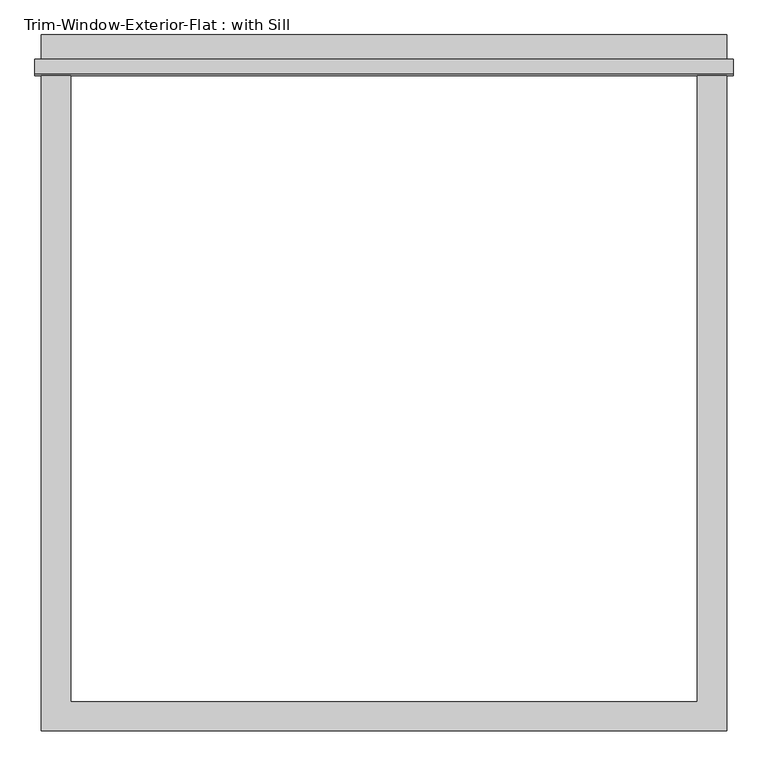
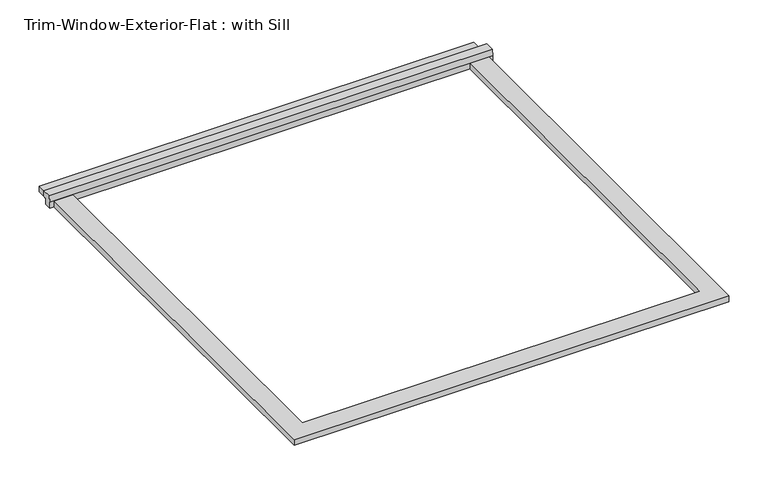
"""IFC4 building model written with IfcOpenShell, lengths in millimetres: proxy geometry, Trim-Window-Exterior-Flat : with Sill."""

from ifc_helpers import new_model, si_unit, frame, origin, origin_with_axes, place, context, project, spatial, polyline, outline, extrude, source, transform, mapped, element, save


def trim_window_exterior_flat_with_sill_ac84ebb5(model_context):
    return source(origin(), model_context, "Body", "SweptSolid", [
        extrude(outline(polyline([(666.75, 1241.3823709), (-666.75, 1241.3823709), (-666.75, 1298.5323709), (666.75, 1298.5323709), (666.75, 1241.3823709)])), origin_with_axes(), (0.0, 0.0, 1.0), 19.05),
        extrude(outline(polyline([(1250.95, 38.1), (1250.95, 19.05), (1241.3823709, 19.05), (1241.3823709, 0.0), (1219.2, 0.0), (1219.2, 19.05), (1221.6580645, 38.1), (1250.95, 38.1)])), frame((-679.45, 0.0, 0.0), z_axis=(1.0, 0.0, 0.0), x_axis=(0.0, 1.0, 0.0)), (0.0, 0.0, 1.0), 1358.9),
        extrude(outline(polyline([(-666.75, -57.15), (-666.75, 1219.2), (-609.6, 1219.2), (-609.6, 0.0), (609.6, 0.0), (609.6, 1219.2), (666.75, 1219.2), (666.75, -57.15), (-666.75, -57.15)])), origin_with_axes(), (0.0, 0.0, 1.0), 19.05),
    ])


if __name__ == "__main__":
    model = new_model("IFC4")
    model_context = context("Model", 3, world=origin())
    ifc_project = project(units=[si_unit("LENGTHUNIT", "METRE", prefix="MILLI")], contexts=[model_context])
    site = spatial("IfcSite", under=ifc_project)
    building = spatial("IfcBuilding", under=site)
    placement = place(None, origin())
    trim_window_exterior_flat_with_sill_shape = trim_window_exterior_flat_with_sill_ac84ebb5(model_context)
    element("IfcBuildingElementProxy", 1, Name="Trim-Window-Exterior-Flat : with Sill", ObjectType="Trim-Window-Exterior-Flat : with Sill", at=placement, inside=building, context=model_context, shape_type="MappedRepresentation", body=[
        mapped(trim_window_exterior_flat_with_sill_shape, transform((0.0, 0.0, 0.0), x_axis=(1.0, 0.0, 0.0), y_axis=(0.0, 1.0, 0.0), z_axis=(0.0, 0.0, 1.0))),
    ])
    save(model, "model.ifc")

# Revit data of these elements
# Type "Trim-Window-Exterior-Flat : with Sill"
#   Trim Width = 0' - 2 1/4"
#   Trim Thickness_Picture Frame = 0' - 1 1/4"
#   Trim Thickness_with Sill = 0' - 0 3/4"
#   Sill Thickness = 0' - 1 1/4"
#   Opening Width [instance default] = 2' - 0"
#   Opening Height [instance default] = 3' - 0"
#   Default Elevation = 4' - 0"
#   Sill = yes
#   Picture Frame = no
#   Trim Material [instance default] = none
# Element 1 (IfcBuildingElementProxy, "Trim-Window-Exterior-Flat : with Sill")
#   Opening Width = 4' - 0"
#   Opening Height = 4' - 0"
#   Trim Material = Clad - White
#   Materials on its faces: "Clad - White"
# Materials
#   "Clad - White": class "Wood", colour RGB 242 242 238, transparency 0, Cost = 0
